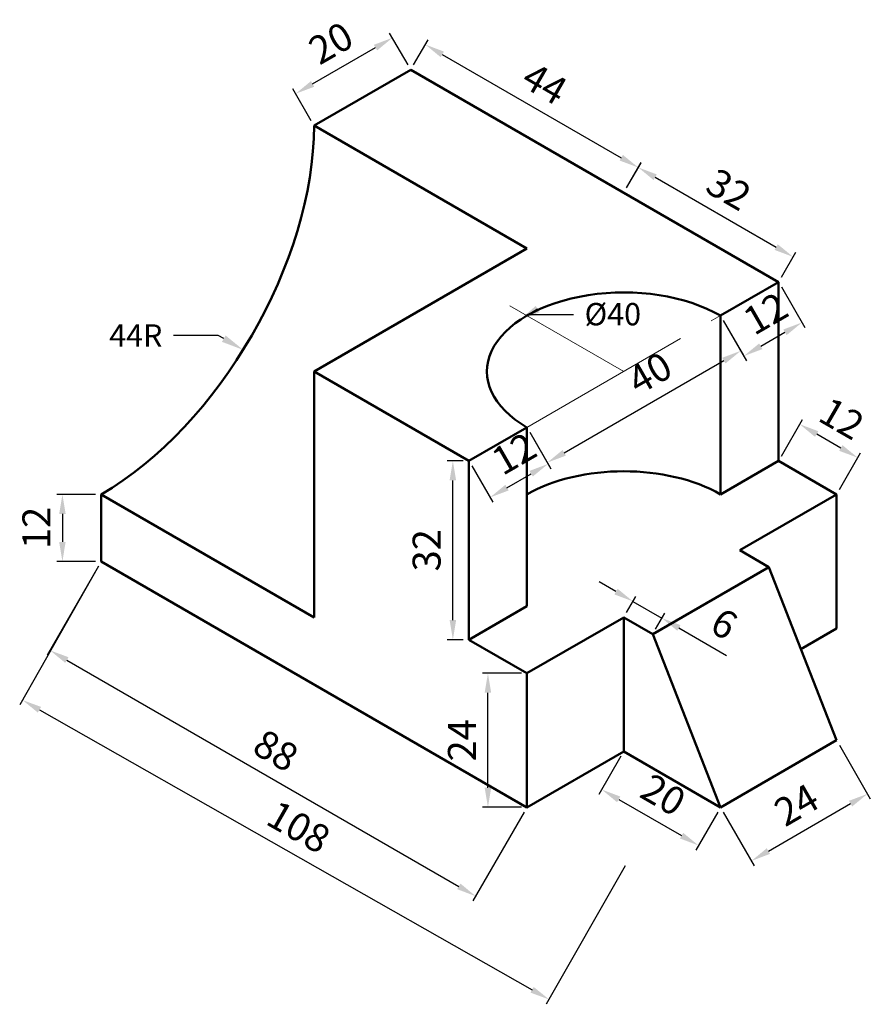
# Model space of a CAD drawing. Units: millimetres. Extents: x 2015 to 2167, y 1477 to 1653.
import ezdxf
from ezdxf import colors
from ezdxf.entities.mleader import LeaderData, LeaderLine
from ezdxf.math import Vec2, Vec3

# ---------------------------------------------------------------- set-up
doc = ezdxf.new("R2010")
doc.units = ezdxf.units.MM
doc.linetypes.add('CENTER', pattern=[50.8, 31.75, -6.35, 6.35, -6.35])
for name, color, linetype, lineweight in [('M-CNTR', 1, 'CENTER', 18), ('M-DIMS', 3, 'Continuous', 25), ('M-OUTL', 7, 'Continuous', 50)]:
    doc.layers.add(name, color=color, linetype=linetype, lineweight=lineweight)
doc.styles.get("Standard").update_dxf_attribs({"font": 'arial.ttf'})
doc.dimstyles.new('AM_ISO$0', dxfattribs={"dimtxt": 5, "dimasz": 3.5, "dimexe": 1, "dimexo": 1, "dimgap": 1.5, "dimtad": 1, "dimdsep": 46, "dimtxsty": 'Standard', "dimcen": 0, "dimclrd": 256, "dimclre": 256, "dimclrt": 2, "dimadec": 0, "dimazin": 2, "dimtp": 0.1, "dimtm": 0.1, "dimtfac": 0.71, "dimtmove": 0, "dimatfit": 3, "dimfxl": 1, "dimlwd": -1, "dimlwe": -1, "dimarcsym": 1})

# ---------------------------------------------------------------- blocks, each defined once
blk = doc.blocks.new('*D3')
at = {"layer": 'Defpoints', "color": 0, "transparency": 16777216}
for p in [(2098.46, 1535.85), (2105.44, 1535.85), (2105.44, 1511.85)]:
    blk.add_point(p, dxfattribs=at)
at = {"layer": 'M-DIMS', "color": 0, "linetype": 'ByBlock', "transparency": 16777216}
for p, q in [((2104.44, 1535.85), (2097.46, 1535.85)), ((2098.46, 1515.35), (2098.46, 1532.35)), ((2104.44, 1511.85), (2097.46, 1511.85))]:
    blk.add_line(p, q, dxfattribs=at)
at = {"layer": 'M-DIMS', "color": 0, "transparency": 16777216}
for points in [[(2097.87, 1532.35), (2099.04, 1532.35), (2098.46, 1535.85)], [(2097.87, 1515.35), (2099.04, 1515.35), (2098.46, 1511.85)]]:
    blk.add_solid(points, dxfattribs=at)
at = {"layer": 'M-DIMS', "color": 0, "transparency": 16777216, "insert": (2094.45, 1523.85), "char_height": 5, "attachment_point": 5, "rotation": 90}
blk.add_mtext('24', dxfattribs=at)
blk = doc.blocks.new('*D4')
at = {"layer": 'Defpoints', "color": 0, "transparency": 16777216}
for p in [(2122.76, 1545.85), (2129.61, 1545.7), (2127.96, 1542.85)]:
    blk.add_point(p, dxfattribs=at)
at = {"layer": 'M-DIMS', "color": 0, "linetype": 'ByBlock', "transparency": 16777216}
for p, q in [((2121.38, 1550.45), (2118.35, 1552.2)), ((2123.26, 1546.71), (2124.91, 1549.57)), ((2124.41, 1548.7), (2129.61, 1545.7)), ((2128.46, 1543.71), (2130.11, 1546.57)), ((2132.64, 1543.95), (2141.13, 1539.05))]:
    blk.add_line(p, q, dxfattribs=at)
at = {"layer": 'M-DIMS', "color": 0, "transparency": 16777216}
for points in [[(2121.67, 1550.96), (2121.09, 1549.95), (2124.41, 1548.7)], [(2132.93, 1544.46), (2132.35, 1543.45), (2129.61, 1545.7)]]:
    blk.add_solid(points, dxfattribs=at)
at = {"layer": 'M-DIMS', "color": 0, "transparency": 16777216, "insert": (2140.43, 1544.14), "char_height": 5, "attachment_point": 5, "rotation": 330}
blk.add_mtext('6', dxfattribs=at)
blk = doc.blocks.new('*D5')
at = {"layer": 'Defpoints', "color": 0, "transparency": 16777216}
for p in [(2122.76, 1521.85), (2140.08, 1511.85), (2136.15, 1505.03)]:
    blk.add_point(p, dxfattribs=at)
at = {"layer": 'M-DIMS', "color": 0, "linetype": 'ByBlock', "transparency": 16777216}
for p, q in [((2122.26, 1520.98), (2118.33, 1514.16)), ((2121.86, 1513.28), (2133.12, 1506.78)), ((2139.58, 1510.98), (2135.65, 1504.16))]:
    blk.add_line(p, q, dxfattribs=at)
at = {"layer": 'M-DIMS', "color": 0, "transparency": 16777216}
for points in [[(2122.15, 1513.78), (2121.57, 1512.77), (2118.83, 1515.03)], [(2133.41, 1507.28), (2132.83, 1506.27), (2136.15, 1505.03)]]:
    blk.add_solid(points, dxfattribs=at)
at = {"layer": 'M-DIMS', "color": 0, "transparency": 16777216, "insert": (2129.52, 1513.54), "char_height": 5, "attachment_point": 5, "rotation": 330}
blk.add_mtext('20', dxfattribs=at)
blk = doc.blocks.new('*D6')
at = {"layer": 'Defpoints', "color": 0, "transparency": 16777216}
for p in [(2029.23, 1567.85), (2022.29, 1555.85), (2029.23, 1555.85)]:
    blk.add_point(p, dxfattribs=at)
at = {"layer": 'M-DIMS', "color": 0, "linetype": 'ByBlock', "transparency": 16777216}
for p, q in [((2028.23, 1567.85), (2021.29, 1567.85)), ((2022.29, 1564.35), (2022.29, 1559.35)), ((2028.23, 1555.85), (2021.29, 1555.85))]:
    blk.add_line(p, q, dxfattribs=at)
at = {"layer": 'M-DIMS', "color": 0, "transparency": 16777216}
for points in [[(2021.71, 1564.35), (2022.87, 1564.35), (2022.29, 1567.85)], [(2021.71, 1559.35), (2022.87, 1559.35), (2022.29, 1555.85)]]:
    blk.add_solid(points, dxfattribs=at)
at = {"layer": 'M-DIMS', "color": 0, "transparency": 16777216, "insert": (2018.28, 1561.85), "char_height": 5, "attachment_point": 5, "rotation": 90}
blk.add_mtext('12', dxfattribs=at)
blk = doc.blocks.new('*D7')
at = {"layer": 'Defpoints', "color": 0, "transparency": 16777216}
for p in [(2105.44, 1579.85), (2095.05, 1573.85), (2109.22, 1573.3)]:
    blk.add_point(p, dxfattribs=at)
at = {"layer": 'M-DIMS', "color": 0, "linetype": 'ByBlock', "transparency": 16777216}
for p, q in [((2105.94, 1578.98), (2109.72, 1572.44)), ((2095.55, 1572.98), (2099.33, 1566.44)), ((2101.86, 1569.05), (2106.19, 1571.55))]:
    blk.add_line(p, q, dxfattribs=at)
at = {"layer": 'M-DIMS', "color": 0, "transparency": 16777216}
for points in [[(2105.9, 1572.06), (2106.48, 1571.05), (2109.22, 1573.3)], [(2101.57, 1569.56), (2102.15, 1568.55), (2098.83, 1567.3)]]:
    blk.add_solid(points, dxfattribs=at)
at = {"layer": 'M-DIMS', "color": 0, "transparency": 16777216, "insert": (2103.44, 1574.6), "char_height": 5, "attachment_point": 5, "rotation": 30}
blk.add_mtext('12', dxfattribs=at)
blk = doc.blocks.new('*D8')
at = {"layer": 'Defpoints', "color": 0, "transparency": 16777216}
for p in [(2150.48, 1605.85), (2140.08, 1599.85), (2154.66, 1598.61)]:
    blk.add_point(p, dxfattribs=at)
at = {"layer": 'M-DIMS', "color": 0, "linetype": 'ByBlock', "transparency": 16777216}
for p, q in [((2150.98, 1604.98), (2155.16, 1597.74)), ((2140.58, 1598.98), (2144.76, 1591.74)), ((2147.29, 1594.36), (2151.62, 1596.86))]:
    blk.add_line(p, q, dxfattribs=at)
at = {"layer": 'M-DIMS', "color": 0, "transparency": 16777216}
for points in [[(2151.33, 1597.36), (2151.92, 1596.35), (2154.66, 1598.61)], [(2147, 1594.86), (2147.59, 1593.85), (2144.26, 1592.61)]]:
    blk.add_solid(points, dxfattribs=at)
at = {"layer": 'M-DIMS', "color": 0, "transparency": 16777216, "insert": (2148.47, 1599.67), "char_height": 5, "attachment_point": 5, "rotation": 30}
blk.add_mtext('12', dxfattribs=at)
blk = doc.blocks.new('*D9')
at = {"layer": 'Defpoints', "color": 0, "transparency": 16777216}
for p in [(2140.08, 1599.85), (2143.72, 1593.54), (2105.44, 1579.85)]:
    blk.add_point(p, dxfattribs=at)
at = {"layer": 'M-DIMS', "color": 0, "linetype": 'ByBlock', "transparency": 16777216}
for p, q in [((2140.58, 1598.98), (2144.22, 1592.68)), ((2112.11, 1575.29), (2140.69, 1591.79)), ((2105.94, 1578.98), (2109.58, 1572.68))]:
    blk.add_line(p, q, dxfattribs=at)
at = {"layer": 'M-DIMS', "color": 0, "transparency": 16777216}
for points in [[(2140.4, 1592.3), (2140.98, 1591.29), (2143.72, 1593.54)], [(2111.82, 1575.8), (2112.41, 1574.79), (2109.08, 1573.54)]]:
    blk.add_solid(points, dxfattribs=at)
at = {"layer": 'M-DIMS', "color": 0, "transparency": 16777216, "insert": (2127.75, 1589), "char_height": 5, "attachment_point": 5, "rotation": 30}
blk.add_mtext('40', dxfattribs=at)
blk = doc.blocks.new('*D10')
at = {"layer": 'Defpoints', "color": 0, "transparency": 16777216}
for p in [(2092.18, 1573.85), (2095.05, 1573.85), (2095.05, 1541.85)]:
    blk.add_point(p, dxfattribs=at)
at = {"layer": 'M-DIMS', "color": 0, "linetype": 'ByBlock', "transparency": 16777216}
for p, q in [((2094.05, 1573.85), (2091.18, 1573.85)), ((2092.18, 1545.35), (2092.18, 1570.35)), ((2094.05, 1541.85), (2091.18, 1541.85))]:
    blk.add_line(p, q, dxfattribs=at)
at = {"layer": 'M-DIMS', "color": 0, "transparency": 16777216}
for points in [[(2091.6, 1570.35), (2092.77, 1570.35), (2092.18, 1573.85)], [(2091.6, 1545.35), (2092.77, 1545.35), (2092.18, 1541.85)]]:
    blk.add_solid(points, dxfattribs=at)
at = {"layer": 'M-DIMS', "color": 0, "transparency": 16777216, "insert": (2088.13, 1557.85), "char_height": 5, "attachment_point": 5, "rotation": 90}
blk.add_mtext('32', dxfattribs=at)
blk = doc.blocks.new('*D11')
at = {"layer": 'Defpoints', "color": 0, "transparency": 16777216}
for p in [(2160.87, 1523.85), (2166.4, 1514.26), (2140.08, 1511.85)]:
    blk.add_point(p, dxfattribs=at)
at = {"layer": 'M-DIMS', "color": 0, "linetype": 'ByBlock', "transparency": 16777216}
for p, q in [((2161.37, 1522.98), (2166.9, 1513.4)), ((2148.65, 1504.01), (2163.37, 1512.51)), ((2140.58, 1510.98), (2146.12, 1501.4))]:
    blk.add_line(p, q, dxfattribs=at)
at = {"layer": 'M-DIMS', "color": 0, "transparency": 16777216}
for points in [[(2163.08, 1513.02), (2163.66, 1512.01), (2166.4, 1514.26)], [(2148.36, 1504.52), (2148.94, 1503.51), (2145.62, 1502.26)]]:
    blk.add_solid(points, dxfattribs=at)
at = {"layer": 'M-DIMS', "color": 0, "transparency": 16777216, "insert": (2154, 1511.74), "char_height": 5, "attachment_point": 5, "rotation": 30}
blk.add_mtext('24', dxfattribs=at)
blk = doc.blocks.new('*D12')
at = {"layer": 'Defpoints', "color": 0, "transparency": 16777216}
for p in [(2150.48, 1573.85), (2164.66, 1574.41), (2160.87, 1567.85)]:
    blk.add_point(p, dxfattribs=at)
at = {"layer": 'M-DIMS', "color": 0, "linetype": 'ByBlock', "transparency": 16777216}
for p, q in [((2150.98, 1574.71), (2154.76, 1581.27)), ((2157.3, 1578.66), (2161.63, 1576.16)), ((2161.37, 1568.71), (2165.16, 1575.27))]:
    blk.add_line(p, q, dxfattribs=at)
at = {"layer": 'M-DIMS', "color": 0, "transparency": 16777216}
for points in [[(2157.59, 1579.16), (2157, 1578.15), (2154.26, 1580.41)], [(2161.92, 1576.66), (2161.33, 1575.65), (2164.66, 1574.41)]]:
    blk.add_solid(points, dxfattribs=at)
at = {"layer": 'M-DIMS', "color": 0, "transparency": 16777216, "insert": (2161.47, 1580.88), "char_height": 5, "attachment_point": 5, "rotation": 330}
blk.add_mtext('12', dxfattribs=at)
blk = doc.blocks.new('*D13')
at = {"layer": 'Defpoints', "color": 0, "transparency": 16777216}
for p in [(2029.23, 1555.85), (2105.44, 1511.85), (2096.27, 1495.95)]:
    blk.add_point(p, dxfattribs=at)
at = {"layer": 'M-DIMS', "color": 0, "linetype": 'ByBlock', "transparency": 16777216}
for p, q in [((2028.73, 1554.98), (2019.56, 1539.09)), ((2023.09, 1538.2), (2093.24, 1497.7)), ((2104.94, 1510.98), (2095.77, 1495.09))]:
    blk.add_line(p, q, dxfattribs=at)
at = {"layer": 'M-DIMS', "color": 0, "transparency": 16777216}
for points in [[(2023.38, 1538.71), (2022.8, 1537.7), (2020.06, 1539.95)], [(2093.53, 1498.21), (2092.95, 1497.2), (2096.27, 1495.95)]]:
    blk.add_solid(points, dxfattribs=at)
at = {"layer": 'M-DIMS', "color": 0, "transparency": 16777216, "insert": (2060.19, 1521.46), "char_height": 5, "attachment_point": 5, "rotation": 330}
blk.add_mtext('88', dxfattribs=at)
blk = doc.blocks.new('*D14')
at = {"layer": 'Defpoints', "color": 0, "transparency": 16777216}
for p in [(2029.23, 1555.85), (2123.5, 1502.27), (2109.4, 1477.47)]:
    blk.add_point(p, dxfattribs=at)
at = {"layer": 'M-DIMS', "color": 0, "linetype": 'ByBlock', "transparency": 16777216}
for p, q in [((2028.74, 1554.98), (2014.64, 1530.18)), ((2018.18, 1529.32), (2106.36, 1479.2)), ((2123, 1501.4), (2108.91, 1476.6))]:
    blk.add_line(p, q, dxfattribs=at)
at = {"layer": 'M-DIMS', "color": 0, "transparency": 16777216}
for points in [[(2018.47, 1529.82), (2017.89, 1528.81), (2015.14, 1531.05)], [(2106.65, 1479.71), (2106.07, 1478.69), (2109.4, 1477.47)]]:
    blk.add_solid(points, dxfattribs=at)
at = {"layer": 'M-DIMS', "color": 0, "transparency": 16777216, "insert": (2064.27, 1507.78), "char_height": 5, "attachment_point": 5, "rotation": 330.3863}
blk.add_mtext('108', dxfattribs=at)
blk = doc.blocks.new('*D15')
at = {"layer": 'Defpoints', "color": 0, "transparency": 16777216}
for p in [(2084.66, 1643.85), (2125.36, 1626.35), (2122.76, 1621.85)]:
    blk.add_point(p, dxfattribs=at)
at = {"layer": 'M-DIMS', "color": 0, "linetype": 'ByBlock', "transparency": 16777216}
for p, q in [((2085.16, 1644.71), (2087.76, 1649.21)), ((2090.29, 1646.6), (2122.33, 1628.1)), ((2123.26, 1622.71), (2125.86, 1627.21))]:
    blk.add_line(p, q, dxfattribs=at)
at = {"layer": 'M-DIMS', "color": 0, "transparency": 16777216}
for points in [[(2090.58, 1647.1), (2090, 1646.09), (2087.26, 1648.35)], [(2122.62, 1628.6), (2122.04, 1627.59), (2125.36, 1626.35)]]:
    blk.add_solid(points, dxfattribs=at)
at = {"layer": 'M-DIMS', "color": 0, "transparency": 16777216, "insert": (2108.31, 1640.81), "char_height": 5, "attachment_point": 5, "rotation": 330}
blk.add_mtext('44', dxfattribs=at)
blk = doc.blocks.new('*D16')
at = {"layer": 'Defpoints', "color": 0, "transparency": 16777216}
for p in [(2122.76, 1621.85), (2153.08, 1610.36), (2150.48, 1605.85)]:
    blk.add_point(p, dxfattribs=at)
at = {"layer": 'M-DIMS', "color": 0, "linetype": 'ByBlock', "transparency": 16777216}
for p, q in [((2123.26, 1622.71), (2125.87, 1627.22)), ((2128.4, 1624.61), (2150.05, 1612.11)), ((2150.98, 1606.71), (2153.58, 1611.22))]:
    blk.add_line(p, q, dxfattribs=at)
at = {"layer": 'M-DIMS', "color": 0, "transparency": 16777216}
for points in [[(2128.69, 1625.11), (2128.11, 1624.1), (2125.37, 1626.36)], [(2150.34, 1612.61), (2149.76, 1611.6), (2153.08, 1610.36)]]:
    blk.add_solid(points, dxfattribs=at)
at = {"layer": 'M-DIMS', "color": 0, "transparency": 16777216, "insert": (2141.25, 1621.87), "char_height": 5, "attachment_point": 5, "rotation": 330}
blk.add_mtext('32', dxfattribs=at)
blk = doc.blocks.new('*D17')
at = {"layer": 'Defpoints', "color": 0, "transparency": 16777216}
for p in [(2081.36, 1649.56), (2084.66, 1643.85), (2067.34, 1633.85)]:
    blk.add_point(p, dxfattribs=at)
at = {"layer": 'M-DIMS', "color": 0, "linetype": 'ByBlock', "transparency": 16777216}
for p, q in [((2084.16, 1644.71), (2080.86, 1650.42)), ((2067.07, 1641.31), (2078.33, 1647.81)), ((2066.84, 1634.71), (2063.54, 1640.42))]:
    blk.add_line(p, q, dxfattribs=at)
at = {"layer": 'M-DIMS', "color": 0, "transparency": 16777216}
for points in [[(2078.04, 1648.31), (2078.62, 1647.3), (2081.36, 1649.56)], [(2066.78, 1641.81), (2067.36, 1640.8), (2064.04, 1639.56)]]:
    blk.add_solid(points, dxfattribs=at)
at = {"layer": 'M-DIMS', "color": 0, "transparency": 16777216, "insert": (2070.67, 1648.07), "char_height": 5, "attachment_point": 5, "rotation": 30}
blk.add_mtext('20', dxfattribs=at)

msp = doc.modelspace()

# ---------------------------------------------------------------- linework, layer by layer
at = {"layer": 'M-CNTR'}
for p, q in [((2122.764, 1589.846), (2102.395, 1601.606)), ((2105.444, 1579.846), (2140.085, 1599.846))]:
    msp.add_line(p, q, dxfattribs=at)
at = {"layer": 'M-OUTL'}
for p, q in [((2084.659, 1643.846), (2067.338, 1633.846)), ((2150.477, 1605.846), (2084.659, 1643.846)), ((2067.338, 1633.846), (2105.444, 1611.846)), ((2067.338, 1589.846), (2105.444, 1611.846)), ((2140.085, 1599.846), (2150.477, 1605.846)), ((2150.477, 1605.846), (2150.477, 1573.846)), ((2140.085, 1567.846), (2140.085, 1599.846)), ((2095.051, 1573.846), (2067.338, 1589.846)), ((2067.338, 1589.846), (2067.338, 1545.846)), ((2105.444, 1579.846), (2095.051, 1573.846)), ((2105.444, 1547.846), (2105.444, 1579.846)), ((2095.051, 1541.846), (2095.051, 1573.846)), ((2150.477, 1573.846), (2140.085, 1567.846)), ((2160.869, 1567.846), (2150.477, 1573.846)), ((2067.338, 1545.846), (2029.233, 1567.846)), ((2029.233, 1555.846), (2029.233, 1567.846)), ((2143.549, 1557.846), (2160.869, 1567.846)), ((2160.869, 1567.846), (2160.869, 1543.846)), ((2143.549, 1557.846), (2148.745, 1554.846)), ((2029.233, 1555.846), (2105.444, 1511.846)), ((2148.745, 1554.846), (2127.96, 1542.846)), ((2148.745, 1554.846), (2160.869, 1523.846)), ((2095.051, 1541.846), (2105.444, 1547.846)), ((2105.444, 1535.846), (2122.764, 1545.846)), ((2122.764, 1545.846), (2122.764, 1521.846)), ((2127.96, 1542.846), (2122.764, 1545.846)), ((2160.869, 1543.846), (2154.488, 1540.162)), ((2105.444, 1535.846), (2095.051, 1541.846)), ((2127.96, 1542.846), (2140.085, 1511.846)), ((2105.444, 1511.846), (2105.444, 1535.846)), ((2140.085, 1511.846), (2160.869, 1523.846)), ((2105.444, 1511.846), (2122.764, 1521.846)), ((2122.764, 1521.846), (2140.085, 1511.846))]:
    msp.add_line(p, q, dxfattribs=at)
for centre, major_axis, start_param, end_param in [((2029.233, 1611.846), (-26.944, -46.669), 0.7853982, 2.3561945), ((2122.764, 1589.846), (-24.495, 0), 3.9269908, 7.0685835), ((2122.764, 1557.846), (-24.495, 0), 3.9269908, 5.4977871)]:
    msp.add_ellipse(centre, major_axis=major_axis, ratio=0.5773503, start_param=start_param, end_param=end_param, dxfattribs=at)

# ---------------------------------------------------------------- dimensions: what is measured, and where the dimension line sits
at = {"layer": 'M-DIMS'}
for p1, p2, distance, override, picture, middle in [((2067.338, 1633.846), (2084.659, 1643.846), 6.595, {"dimpost": '', "dimclrd": 0, "dimclre": 0, "dimclrt": 0}, '*D17', (2070.675, 1648.067)), ((2084.659, 1643.846), (2122.764, 1621.846), 5.196, {"dimpost": '', "dimclrd": 0, "dimclre": 0, "dimclrt": 0}, '*D15', (2108.31, 1640.81)), ((2150.477, 1573.846), (2160.869, 1567.846), 7.575, {"dimpost": '', "dimclrd": 0, "dimclre": 0, "dimclrt": 0}, '*D12', (2161.466, 1580.879)), ((2095.051, 1541.846), (2095.051, 1573.846), 2.868, {"dimpost": '', "dimclrd": 0, "dimclre": 0, "dimclrt": 0}, '*D10', (2088.129, 1557.846)), ((2029.233, 1567.846), (2029.233, 1555.846), -6.943, {"dimclrd": 0, "dimclre": 0, "dimclrt": 0}, '*D6', (2018.28, 1561.846)), ((2029.233, 1555.846), (2105.444, 1511.846), -18.35, {"dimclrd": 0, "dimclre": 0, "dimclrt": 0}, '*D13', (2060.19, 1521.464)), ((2122.764, 1545.846), (2127.96, 1542.846), 3.298, {"dimclrd": 0, "dimclre": 0, "dimclrt": 0}, '*D4', (2140.427, 1544.137)), ((2105.444, 1511.846), (2105.444, 1535.846), 6.988, {"dimclrd": 0, "dimclre": 0, "dimclrt": 0}, '*D3', (2094.445, 1523.846)), ((2122.764, 1521.846), (2140.085, 1511.846), -7.871, {"dimclrd": 0, "dimclre": 0, "dimclrt": 0}, '*D5', (2129.515, 1513.539))]:
    dim = msp.add_aligned_dim(p1=p1, p2=p2, distance=distance, dimstyle='AM_ISO$0', override=override, dxfattribs=at)
    dim.commit()
    dim.dimension.update_dxf_attribs({"geometry": picture, "text_midpoint": middle})
for base, p1, p2, angle, picture, middle in [((2153.08, 1610.355), (2122.764, 1621.846), (2150.477, 1605.846), 330, '*D16', (2139.224, 1618.355)), ((2154.655, 1598.608), (2140.085, 1599.846), (2150.477, 1605.846), 30, '*D8', (2150.477, 1596.196)), ((2143.724, 1593.542), (2105.444, 1579.846), (2140.085, 1599.846), 30, '*D9', (2129.781, 1585.492)), ((2109.221, 1573.303), (2095.051, 1573.846), (2105.444, 1579.846), 30, '*D7', (2105.444, 1571.122)), ((2166.402, 1514.264), (2140.085, 1511.846), (2160.869, 1523.846), 30, '*D11', (2156.009, 1508.264))]:
    dim = msp.add_linear_dim(base=base, p1=p1, p2=p2, angle=angle, dimstyle='AM_ISO$0', override={"dimclrd": 0, "dimclre": 0, "dimclrt": 0}, dxfattribs=at)
    dim.commit()
    dim.dimension.update_dxf_attribs({"geometry": picture, "text_midpoint": middle, "dimtype": 161})
dim = msp.add_aligned_dim(p1=(2029.233, 1555.846), p2=(2123.495, 1502.268), distance=-28.525, text='108', dimstyle='AM_ISO$0', override={"dimpost": '', "dimclrd": 0, "dimclre": 0, "dimclrt": 0}, dxfattribs=at)
dim.commit()
dim.dimension.update_dxf_attribs({"geometry": '*D14', "text_midpoint": (2064.271, 1507.782)})

# ---------------------------------------------------------------- leaders
ml = msp.add_multileader_mtext('Standard', dxfattribs=at)
ml.set_content('{\\C2;%%C40}', color=256)
ml.set_leader_properties()
ml.build(insert=Vec2(0, 0))
ctx = ml.context
ctx.base_point, ctx.plane_origin = Vec3(2113.757, 1600.023), Vec3(2103.955, 1598.905)
notes = []
notes.append((ctx, [(0, (1, 1, 0), (2105.757, 1600.023), (1, 0), 8, [(0, [(2103.955, 1598.905)], 0, [])])]))
ctx.mtext.insert, ctx.mtext.flow_direction = Vec3(2115.757, 1602.104), 5
ml = msp.add_multileader_mtext('Standard', dxfattribs=at)
ml.set_content('{\\C2;44R}', color=256)
ml.set_leader_properties()
ml.build(insert=Vec2(0, 0))
ctx = ml.context
ctx.base_point, ctx.plane_origin = Vec3(2028.078, 1596.29), Vec3(2054.639, 1593.72)
ctx.text_align_type = 2
notes.append((ctx, [(0, (1, 1, 0), (2050.188, 1596.29), (-1, 0), 8, [(0, [(2054.639, 1593.72)], 0, [])])]))
ctx.mtext.insert, ctx.mtext.alignment, ctx.mtext.flow_direction = Vec3(2040.188, 1598.29), 3, 5
for ctx, leaders in notes:
    for number, flags, end, landing, length, lines in leaders:
        leader = LeaderData()
        leader.index, (leader.has_last_leader_line, leader.has_dogleg_vector, leader.attachment_direction) = number, flags
        leader.last_leader_point, leader.dogleg_vector, leader.dogleg_length = Vec3(end), Vec3(landing), length
        for number, points, colour, breaks in lines:
            line = LeaderLine()
            line.index, line.vertices, line.color, line.breaks = number, Vec3.list(points), colors.encode_raw_color(colour), breaks
            leader.lines.append(line)
        ctx.leaders.append(leader)

doc.saveas('drawing.dxf')
